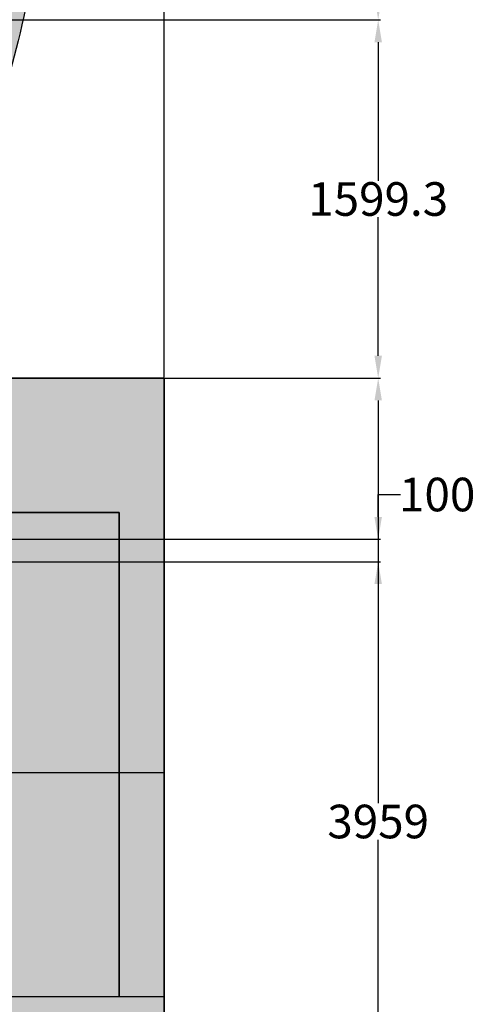
# Model space of a CAD drawing. Units: millimetres. Extents: x 11032 to 26788, y 3406 to 24505.
# Tile 70 of 78: x 24753 to 26788, y 8325 to 12721. Entities that reach past the tile are written whole.
import ezdxf

# ---------------------------------------------------------------- set-up
doc = ezdxf.new("R2010")
doc.units = ezdxf.units.MM
doc.header["$MEASUREMENT"] = 0
for name, color, linetype, lineweight in [('A-ANNO-DIMS', 2, 'Continuous', 18), ('A-FLOR-STRS', 7, 'Continuous', 25), ('A-FLOR-STRS-PATT', 8, 'Continuous', 13), ('A-ROOF', 7, 'Continuous', 30), ('A-WALL', 7, 'Continuous', 35)]:
    doc.layers.add(name, color=color, linetype=linetype, lineweight=lineweight)
doc.layers.add('A-ROOF-PATT', color=9, linetype='Continuous', lineweight=13, true_color=0xc7c8ca)
doc.layers.add('A-WALL-CLAD-PATT', color=9, linetype='Continuous', lineweight=13, true_color=0xc7c8ca)
doc.styles.get("Standard").update_dxf_attribs({"font": 'arial.ttf'})
doc.dimstyles.get("Standard").update_dxf_attribs({"dimtxt": 150, "dimasz": 100, "dimexe": 10, "dimexo": 5, "dimgap": 5, "dimtad": 0, "dimtih": 1, "dimtoh": 1, "dimdec": 0, "dimzin": 0, "dimdsep": 46, "dimtxsty": 'Standard', "dimcen": 0.09, "dimadec": 0, "dimazin": 0, "dimtfac": 1, "dimtdec": 0, "dimtofl": 0, "dimtmove": 0, "dimatfit": 3, "dimfxl": 1, "dimtolj": 1, "dimtzin": 0, "dimarcsym": 0})

# ---------------------------------------------------------------- blocks, each defined once
blk = doc.blocks.new('*D36')
at = {"layer": 'A-ANNO-DIMS', "color": 0, "lineweight": -2, "transparency": 16777216}
for p, q in [((12301.3, 17115.9), (12301.3, 24416.9)), ((12401.3, 24406.9), (18569.2, 24406.9)), ((25297.4, 24406.9), (19129.5, 24406.9)), ((25397.4, 4466.4), (25397.4, 24416.9))]:
    blk.add_line(p, q, dxfattribs=at)
at = {"layer": 'A-ANNO-DIMS', "color": 0, "transparency": 16777216}
for points in [[(12401.3, 24423.5), (12401.3, 24390.2), (12301.3, 24406.9)], [(25297.4, 24423.5), (25297.4, 24390.2), (25397.4, 24406.9)]]:
    blk.add_solid(points, dxfattribs=at)
at = {"layer": 'Defpoints', "color": 0, "transparency": 16777216}
for p in [(25397.4, 24406.9), (12301.3, 17110.9), (25397.4, 4461.4)]:
    blk.add_point(p, dxfattribs=at)
at = {"layer": 'A-ANNO-DIMS', "color": 0, "transparency": 16777216, "insert": (18849.3, 24406.9), "char_height": 150, "attachment_point": 5}
blk.add_mtext('\\A1;13096', dxfattribs=at)
blk = doc.blocks.new('*D40')
at = {"layer": 'A-ANNO-DIMS', "color": 0, "lineweight": -2, "transparency": 16777216}
for p, q in [((25402.4, 11120.8), (26363.9, 11120.8)), ((26353.9, 11020.8), (26353.9, 9222.7)), ((26353.9, 7261.4), (26353.9, 9059.4)), ((25402.4, 7161.4), (26363.9, 7161.4))]:
    blk.add_line(p, q, dxfattribs=at)
at = {"layer": 'A-ANNO-DIMS', "color": 0, "transparency": 16777216}
for points in [[(26337.2, 11020.8), (26370.6, 11020.8), (26353.9, 11120.8)], [(26337.2, 7261.4), (26370.6, 7261.4), (26353.9, 7161.4)]]:
    blk.add_solid(points, dxfattribs=at)
at = {"layer": 'Defpoints', "color": 0, "transparency": 16777216}
for p in [(25397.4, 11120.8), (26353.9, 11120.8), (25397.4, 7161.4)]:
    blk.add_point(p, dxfattribs=at)
at = {"layer": 'A-ANNO-DIMS', "color": 0, "transparency": 16777216, "insert": (26353.9, 9141.1), "char_height": 150, "attachment_point": 5}
blk.add_mtext('\\A1;3959', dxfattribs=at)
blk = doc.blocks.new('*D41')
at = {"layer": 'A-ANNO-DIMS', "color": 0, "lineweight": -2, "transparency": 16777216}
for p, q in [((22752.4, 12720.1), (26363.9, 12720.1)), ((26353.9, 12620.1), (26353.9, 12002)), ((26353.9, 11220.8), (26353.9, 11838.8)), ((25402.4, 11120.8), (26363.9, 11120.8))]:
    blk.add_line(p, q, dxfattribs=at)
at = {"layer": 'A-ANNO-DIMS', "color": 0, "transparency": 16777216}
for points in [[(26337.2, 12620.1), (26370.6, 12620.1), (26353.9, 12720.1)], [(26337.2, 11220.8), (26370.6, 11220.8), (26353.9, 11120.8)]]:
    blk.add_solid(points, dxfattribs=at)
at = {"layer": 'Defpoints', "color": 0, "transparency": 16777216}
for p in [(22747.4, 12720.1), (26353.9, 12720.1), (25397.4, 11120.8)]:
    blk.add_point(p, dxfattribs=at)
at = {"layer": 'A-ANNO-DIMS', "color": 0, "transparency": 16777216, "insert": (26353.9, 11920.4), "char_height": 150, "attachment_point": 5}
blk.add_mtext('\\A1;1599.3', dxfattribs=at)
blk = doc.blocks.new('*D42')
at = {"layer": 'A-ANNO-DIMS', "color": 0, "lineweight": -2, "transparency": 16777216}
for p, q in [((22752.4, 13320.1), (26363.9, 13320.1)), ((26353.9, 13220.1), (26353.9, 13101.7)), ((26353.9, 12820.1), (26353.9, 12938.5)), ((22752.4, 12720.1), (26363.9, 12720.1))]:
    blk.add_line(p, q, dxfattribs=at)
at = {"layer": 'A-ANNO-DIMS', "color": 0, "transparency": 16777216}
for points in [[(26337.2, 13220.1), (26370.6, 13220.1), (26353.9, 13320.1)], [(26337.2, 12820.1), (26370.6, 12820.1), (26353.9, 12720.1)]]:
    blk.add_solid(points, dxfattribs=at)
at = {"layer": 'Defpoints', "color": 0, "transparency": 16777216}
for p in [(22747.4, 13320.1), (26353.9, 13320.1), (22747.4, 12720.1)]:
    blk.add_point(p, dxfattribs=at)
at = {"layer": 'A-ANNO-DIMS', "color": 0, "transparency": 16777216, "insert": (26353.9, 13020.1), "char_height": 150, "attachment_point": 5}
blk.add_mtext('\\A1;600', dxfattribs=at)
blk = doc.blocks.new('*D53')
at = {"layer": 'A-ANNO-DIMS', "color": 0, "lineweight": -2, "transparency": 16777216}
for p, q in [((22897.4, 11115.8), (22897.4, 3494.9)), ((25397.4, 11115.8), (25397.4, 3494.9)), ((22997.4, 3504.9), (23917.4, 3504.9)), ((25297.4, 3504.9), (24377.4, 3504.9))]:
    blk.add_line(p, q, dxfattribs=at)
at = {"layer": 'A-ANNO-DIMS', "color": 0, "transparency": 16777216}
for points in [[(22997.4, 3521.6), (22997.4, 3488.2), (22897.4, 3504.9)], [(25297.4, 3521.6), (25297.4, 3488.2), (25397.4, 3504.9)]]:
    blk.add_solid(points, dxfattribs=at)
at = {"layer": 'Defpoints', "color": 0, "transparency": 16777216}
for p in [(22897.4, 11120.8), (25397.4, 11120.8), (25397.4, 3504.9)]:
    blk.add_point(p, dxfattribs=at)
at = {"layer": 'A-ANNO-DIMS', "color": 0, "transparency": 16777216, "insert": (24147.4, 3504.9), "char_height": 150, "attachment_point": 5}
blk.add_mtext('\\A1;2500', dxfattribs=at)
blk = doc.blocks.new('*D68')
at = {"layer": 'A-ANNO-DIMS', "color": 0, "lineweight": -2, "transparency": 16777216}
for p, q in [((26353.9, 10501), (26353.9, 10601)), ((26353.9, 10601), (26453.9, 10601)), ((16730.9, 10401), (26363.9, 10401)), ((16730.9, 10301), (26363.9, 10301)), ((26353.9, 10201), (26353.9, 10101))]:
    blk.add_line(p, q, dxfattribs=at)
at = {"layer": 'A-ANNO-DIMS', "color": 0, "transparency": 16777216}
for points in [[(26337.2, 10501), (26370.6, 10501), (26353.9, 10401)], [(26337.2, 10201), (26370.6, 10201), (26353.9, 10301)]]:
    blk.add_solid(points, dxfattribs=at)
at = {"layer": 'Defpoints', "color": 0, "transparency": 16777216}
for p in [(16725.9, 10401), (26353.9, 10401), (16725.9, 10301)]:
    blk.add_point(p, dxfattribs=at)
at = {"layer": 'A-ANNO-DIMS', "color": 0, "transparency": 16777216, "insert": (26617.3, 10601), "char_height": 150, "attachment_point": 5}
blk.add_mtext('\\A1;100', dxfattribs=at)

msp = doc.modelspace()

# ---------------------------------------------------------------- hatches: boundary and pattern name
at = {"layer": 'A-FLOR-STRS-PATT'}
h = msp.add_hatch(color=256, dxfattribs=at)
h.set_gradient(color1=(254, 204, 102), color2=(254, 234, 185), name='CURVED')
h.paths.add_polyline_path([(24697.404, 9359.601), (25197.404, 9359.601), (25197.404, 10520.753), (24697.404, 10520.753)])
h = msp.add_hatch(color=256, dxfattribs=at)
h.paths.add_polyline_path([(25197.404, 9359.601), (24697.404, 9359.601), (24697.404, 8359.601), (25197.404, 8359.601)])
h.paths.add_polyline_path([(25397.404, 9359.601), (25197.404, 9359.601), (25197.404, 8359.601), (25397.404, 8359.601)])
h = msp.add_hatch(color=256, dxfattribs=at)
h.set_gradient(color1=(99, 100, 102), color2=(199, 200, 202), name='INVCYLINDER')
edge = h.paths.add_edge_path()
edge.add_line((25397.404, 7412.598), (25397.404, 7559.601))
edge.add_line((25397.404, 7559.601), (23046.275, 7559.601))
edge.add_spline(control_points=[(23046.275, 7559.601), (23037.048, 7510.534), (23026.981, 7461.537), (23016.203, 7412.598)], knot_values=[4765.18021096, 4765.18021096, 4765.18021096, 4765.18021096, 4915.21350677, 4915.21350677, 4915.21350677, 4915.21350677], degree=3, periodic=0)
edge.add_line((23016.203, 7412.598), (25397.404, 7412.598))
edge = h.paths.add_edge_path()
edge.add_line((25397.404, 7759.601), (25397.404, 7959.601))
edge.add_line((25397.404, 7959.601), (23100.115, 7959.601))
edge.add_spline(control_points=[(23100.115, 7959.601), (23095.091, 7892.764), (23087.893, 7826.106), (23078.842, 7759.601)], knot_values=[4359.24967367, 4359.24967367, 4359.24967367, 4359.24967367, 4561.7478912, 4561.7478912, 4561.7478912, 4561.7478912], degree=3, periodic=0)
edge.add_line((23078.842, 7759.601), (25397.404, 7759.601))
h.paths.add_polyline_path([(25397.404, 8159.601), (25397.404, 8359.601), (23721.755, 8359.601), (23721.613, 8159.601)])
at = {"layer": 'A-ROOF-PATT'}
h = msp.add_hatch(color=256, dxfattribs=at)
h.set_gradient(color1=(254, 234, 185), color2=(254, 204, 102), name='HEMISPHERICAL')
edge = h.paths.add_edge_path()
edge.add_spline(control_points=[(22897.404, 11669.966), (22905.925, 11665.421), (23315.936, 11448.075), (24040.798, 11159.928), (24591.756, 12047.169), (24823.737, 12810.982), (24947.403, 13888.961), (24865.187, 14241.353)], knot_values=[3287.74811127, 3287.74811127, 3287.74811127, 3287.74811127, 3313.95061448, 4543.69878516, 5160.49832431, 6201.61230094, 7164.26935092, 7164.26935092, 7164.26935092, 7164.26935092], degree=3, periodic=0)
edge.add_spline(control_points=[(24865.187, 14241.353), (24864.423, 14242.575), (24766.311, 14398.016), (24602.876, 14465.087), (24430.499, 14490.269)], knot_values=[2462.20964139, 2462.20964139, 2462.20964139, 2462.20964139, 2466.8266732, 3052.28296943, 3052.28296943, 3052.28296943, 3052.28296943], degree=3, periodic=0)
edge.add_spline(control_points=[(24430.499, 14490.269), (24425.883, 14491.82), (24421.191, 14493.323), (24402.038, 14499.174), (24386.985, 14503.129), (24351.089, 14511.181), (24329.855, 14514.969), (24285.944, 14521.074), (24263.27, 14523.392), (24216.998, 14526.696), (24193.401, 14527.682), (24156.534, 14528.34), (24143.408, 14528.404), (24117.112, 14528.234), (24103.938, 14528.001), (24070.613, 14527.088), (24050.758, 14526.245), (24021.415, 14524.553), (24011.706, 14523.918), (23966.994, 14520.648), (23932.846, 14517.154), (23866.075, 14508.38), (23833.453, 14503.099), (23769.399, 14490.798), (23737.967, 14483.778), (23675.954, 14468.02), (23645.373, 14459.282), (23584.735, 14440.092), (23554.677, 14429.638), (23494.779, 14407.002), (23464.938, 14394.819), (23420.13, 14375.236), (23405.186, 14368.49), (23382.735, 14358.043), (23375.245, 14354.506), (23363.999, 14349.118), (23360.248, 14347.308), (23354.645, 14344.586), (23352.794, 14343.684), (23350.017, 14342.326), (23349.099, 14341.876), (23346.705, 14340.7), (23345.24, 14339.978), (23338.743, 14336.765), (23333.903, 14334.336), (23322.952, 14328.714), (23316.906, 14325.517), (23304.544, 14318.72), (23298.224, 14315.118), (23284.755, 14307.106), (23277.606, 14302.694), (23262.032, 14292.682), (23253.61, 14287.081), (23235.154, 14274.351), (23225.122, 14267.224), (23200.911, 14249.486), (23186.304, 14238.46), (23150.266, 14210.435), (23128.041, 14192.649), (23080.227, 14153.32), (23055.083, 14132.223), (23027.357, 14108.523)], knot_values=[765.02120011, 765.02120011, 765.02120011, 765.02120011, 788.26421035, 788.26421035, 858.47024111, 858.47024111, 949.55129088, 949.55129088, 1040.63234064, 1040.63234064, 1131.71339041, 1131.71339041, 1181.69353236, 1181.69353236, 1231.67367431, 1231.67367431, 1308.31901537, 1308.31901537, 1346.64168591, 1346.64168591, 1486.09404767, 1486.09404767, 1625.54640943, 1625.54640943, 1764.99877119, 1764.99877119, 1904.45113295, 1904.45113295, 2043.90349471, 2043.90349471, 2183.35585648, 2183.35585648, 2253.08203736, 2253.08203736, 2287.9451278, 2287.9451278, 2305.37667302, 2305.37667302, 2313.97014819, 2313.97014819, 2318.26688578, 2318.26688578, 2325.26983634, 2325.26983634, 2349.68341829, 2349.68341829, 2381.60377634, 2381.60377634, 2413.52413439, 2413.52413439, 2445.44449243, 2445.44449243, 2477.36485048, 2477.36485048, 2509.28520853, 2509.28520853, 2547.80727814, 2547.80727814, 2595.07704725, 2595.07704725, 2638.35089074, 2638.35089074, 2638.35089074, 2638.35089074], degree=3, periodic=0)
edge.add_spline(control_points=[(23027.357, 14108.523), (23027.349, 14108.516), (23027.342, 14108.51), (23027.334, 14108.504), (22984.024, 14071.482), (22940.714, 14034.46), (22897.404, 13997.439)], knot_values=[697.41436256, 697.41436256, 697.41436256, 697.41436256, 697.4261083, 697.4261083, 697.4261083, 765.02120011, 765.02120011, 765.02120011, 765.02120011], degree=3, periodic=0)
edge.add_line((22897.404, 13997.439), (22897.404, 11669.966))
h.paths.add_polyline_path([(23729.349, 12537.488, -1), (23529.349, 12537.488, -1)], flags=16)
h.paths.add_polyline_path([(23963.611, 13699.89, -1), (24163.611, 13699.89, -1)], flags=16)
at = {"layer": 'A-WALL-CLAD-PATT'}
h = msp.add_hatch(color=256, dxfattribs=at)
edge = h.paths.add_edge_path()
edge.add_spline(control_points=[(24865.187, 14241.353), (24844.683, 14329.238), (24708.481, 14689.762), (23980.011, 14777.842), (23439.65, 14624.598), (23111.535, 14443.589), (22897.404, 14260.55)], knot_values=[765.02120011, 765.02120011, 765.02120011, 765.02120011, 1005.10337375, 1880.54593672, 2963.32805357, 3287.74811127, 3287.74811127, 3287.74811127, 3287.74811127], degree=3, periodic=0)
edge.add_line((22897.404, 14260.55), (22897.404, 13997.439))
edge.add_spline(control_points=[(22897.404, 13997.439), (22940.714, 14034.46), (22984.024, 14071.482), (23027.334, 14108.504), (23027.342, 14108.51), (23027.349, 14108.516), (23027.357, 14108.523)], knot_values=[697.41436256, 697.41436256, 697.41436256, 697.41436256, 765.00945437, 765.00945437, 765.00945437, 765.02120011, 765.02120011, 765.02120011, 765.02120011], degree=3, periodic=0)
edge.add_spline(control_points=[(23027.357, 14108.523), (23055.083, 14132.223), (23080.227, 14153.32), (23128.041, 14192.649), (23150.266, 14210.435), (23186.304, 14238.46), (23200.911, 14249.486), (23225.122, 14267.224), (23235.154, 14274.351), (23253.61, 14287.081), (23262.032, 14292.682), (23277.606, 14302.694), (23284.755, 14307.106), (23298.224, 14315.118), (23304.544, 14318.72), (23316.906, 14325.517), (23322.952, 14328.714), (23333.903, 14334.336), (23338.743, 14336.765), (23345.24, 14339.978), (23346.705, 14340.7), (23349.099, 14341.876), (23350.017, 14342.326), (23352.794, 14343.684), (23354.645, 14344.586), (23360.248, 14347.308), (23363.999, 14349.118), (23375.245, 14354.506), (23382.735, 14358.043), (23405.186, 14368.49), (23420.13, 14375.236), (23464.938, 14394.819), (23494.779, 14407.002), (23554.677, 14429.638), (23584.735, 14440.092), (23645.373, 14459.282), (23675.954, 14468.02), (23737.967, 14483.778), (23769.399, 14490.798), (23833.453, 14503.099), (23866.075, 14508.38), (23932.846, 14517.154), (23966.994, 14520.648), (24011.706, 14523.918), (24021.415, 14524.553), (24050.758, 14526.245), (24070.613, 14527.088), (24103.938, 14528.001), (24117.112, 14528.234), (24143.408, 14528.404), (24156.534, 14528.34), (24193.401, 14527.682), (24216.998, 14526.696), (24263.27, 14523.392), (24285.944, 14521.074), (24329.855, 14514.969), (24351.089, 14511.181), (24386.985, 14503.129), (24402.038, 14499.174), (24421.191, 14493.323), (24425.883, 14491.82), (24430.499, 14490.269)], knot_values=[765.02120011, 765.02120011, 765.02120011, 765.02120011, 808.29504361, 808.29504361, 855.56481272, 855.56481272, 894.08688233, 894.08688233, 926.00724037, 926.00724037, 957.92759842, 957.92759842, 989.84795647, 989.84795647, 1021.76831451, 1021.76831451, 1053.68867256, 1053.68867256, 1078.10225451, 1078.10225451, 1085.10520508, 1085.10520508, 1089.40194266, 1089.40194266, 1097.99541784, 1097.99541784, 1115.42696306, 1115.42696306, 1150.2900535, 1150.2900535, 1220.01623438, 1220.01623438, 1359.46859614, 1359.46859614, 1498.9209579, 1498.9209579, 1638.37331966, 1638.37331966, 1777.82568142, 1777.82568142, 1917.27804319, 1917.27804319, 2056.73040495, 2056.73040495, 2095.05307548, 2095.05307548, 2171.69841654, 2171.69841654, 2221.67855849, 2221.67855849, 2271.65870045, 2271.65870045, 2362.73975021, 2362.73975021, 2453.82079998, 2453.82079998, 2544.90184974, 2544.90184974, 2615.10788051, 2615.10788051, 2638.35089074, 2638.35089074, 2638.35089074, 2638.35089074], degree=3, periodic=0)
edge.add_spline(control_points=[(24430.499, 14490.269), (24602.876, 14465.087), (24766.311, 14398.016), (24864.423, 14242.575), (24865.187, 14241.353)], knot_values=[2462.20964139, 2462.20964139, 2462.20964139, 2462.20964139, 3047.66593763, 3052.28296943, 3052.28296943, 3052.28296943, 3052.28296943], degree=3, periodic=0)
h.paths.add_polyline_path([(25397.404, 11120.753), (22897.404, 11120.753), (22897.404, 10520.753), (25197.404, 10520.753), (25197.404, 9359.601), (25397.404, 9359.601)])

# ---------------------------------------------------------------- linework, layer by layer
at = {"layer": 'A-FLOR-STRS'}
for p, q in [((24697.404, 9359.601), (25397.404, 9359.601)), ((23721.755, 8359.601), (25397.404, 8359.601))]:
    msp.add_line(p, q, dxfattribs=at)
at = {"layer": 'A-ROOF'}
msp.add_open_spline([(22897.404, 14260.55), (23111.535, 14443.589), (23439.65, 14624.598), (23980.011, 14777.842), (25027.484, 14651.191), (24844.989, 12880.959), (24591.756, 12047.169), (24040.798, 11159.928), (23315.936, 11448.075), (22905.925, 11665.421), (22897.404, 11669.966)], degree=3, knots=[765.02120011, 765.02120011, 765.02120011, 765.02120011, 1089.44125781, 2172.22337467, 3047.66593763, 4250.40516126, 5291.51913789, 5908.31867703, 7138.06684772, 7164.26935092, 7164.26935092, 7164.26935092, 7164.26935092], dxfattribs=at)
at = {"layer": 'A-WALL'}
for p, q in [((22897.404, 11120.753), (25397.404, 11120.753)), ((25397.404, 11120.753), (25397.404, 7161.399)), ((22897.404, 10520.753), (25197.404, 10520.753)), ((25197.404, 10520.753), (25197.404, 8359.601))]:
    msp.add_line(p, q, dxfattribs=at)

# ---------------------------------------------------------------- dimensions: what is measured, and where the dimension line sits
at = {"layer": 'A-ANNO-DIMS'}
for base, p1, p2, picture, middle in [((25397.404, 24406.858), (12301.265, 17110.885), (25397.404, 4461.399), '*D36', (18849.334, 24406.858)), ((25397.404, 3504.899), (22897.404, 11120.753), (25397.404, 11120.753), '*D53', (24147.404, 3504.899))]:
    dim = msp.add_linear_dim(base=base, p1=p1, p2=p2, dimstyle='Standard', override={"dimdec": 0, "dimlfac": 1, "dimrnd": 0, "dimzin": 0, "dimdsep": 46, "dimlunit": 2}, dxfattribs=at)
    dim.commit()
    dim.dimension.update_dxf_attribs({"geometry": picture, "text_midpoint": middle})
for base, p1, p2, override, picture, middle in [((26353.904, 13320.07), (22747.404, 12720.064), (22747.404, 13320.07), {"dimdec": 0, "dimlfac": 1, "dimrnd": 0, "dimzin": 0, "dimdsep": 46, "dimlunit": 2}, '*D42', (26353.904, 13020.067)), ((26353.904, 12720.064), (25397.404, 11120.753), (22747.404, 12720.064), {"dimdec": 1, "dimlfac": 1, "dimrnd": 0, "dimzin": 0, "dimdsep": 46, "dimlunit": 2}, '*D41', (26353.904, 11920.409)), ((26353.904, 11120.753), (25397.404, 7161.399), (25397.404, 11120.753), {"dimdec": 0, "dimlfac": 1, "dimrnd": 0, "dimzin": 0, "dimdsep": 46, "dimlunit": 2}, '*D40', (26353.904, 9141.076)), ((26353.904, 10401.016), (16725.949, 10301.016), (16725.949, 10401.016), {"dimdec": 0, "dimlfac": 1, "dimrnd": 0, "dimzin": 0, "dimdsep": 46, "dimlunit": 2}, '*D68', (26617.294, 10601.016))]:
    dim = msp.add_linear_dim(base=base, p1=p1, p2=p2, angle=90, dimstyle='Standard', override=override, dxfattribs=at)
    dim.commit()
    dim.dimension.update_dxf_attribs({"geometry": picture, "text_midpoint": middle})

doc.saveas('drawing.dxf')
